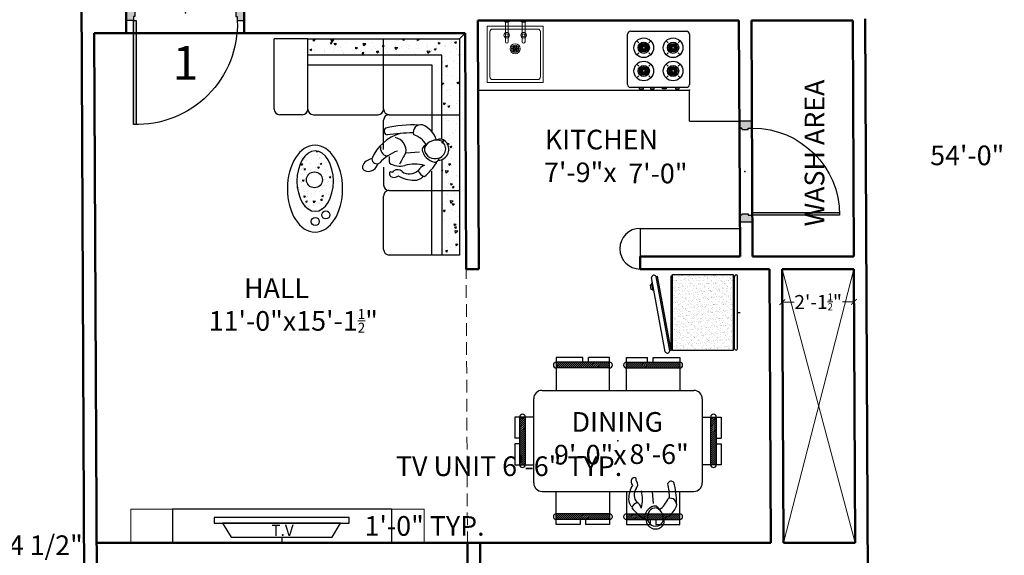
# Model space of a CAD drawing. Units: inches. Extents: x 4508 to 5907, y 877 to 1592.
# Tile 14 of 20: x 5553 to 5904, y 1107 to 1298. Entities that reach past the tile are written whole.
import ezdxf

# ---------------------------------------------------------------- set-up
doc = ezdxf.new("R2010")
doc.units = ezdxf.units.IN
doc.linetypes.add('DASHED', pattern=[0.75, 0.5, -0.25])
doc.layers.get('DEFPOINTS').update_dxf_attribs({"color": 8})
for name, color, linetype, lineweight in [('A-ANNO-DIMS', 2, 'Continuous', 18), ('A-ANNO-TEXT', 7, 'Continuous', 25), ('A-DOOR', 4, 'Continuous', 25), ('A-FLOR-CASE', 30, 'Continuous', 25), ('A-FLOR-FIXT', 8, 'Continuous', 18), ('A-FLOR-OVHD', 5, 'DASHED', 18), ('A-FLOR-SHFT', 8, 'Continuous', 18), ('A-FURN', 24, 'Continuous', 18), ('A-WALL', 7, 'Continuous', 50)]:
    doc.layers.add(name, color=color, linetype=linetype, lineweight=lineweight)
doc.layers.add('doors & windows', color=30, linetype='Continuous')
doc.layers.add('furniture', color=24, linetype='Continuous')
doc.styles.get("Standard").update_dxf_attribs({"font": 'arial.ttf'})
doc.dimstyles.new('details', dxfattribs={"dimtxt": 5, "dimasz": 2, "dimexe": 2, "dimexo": 3, "dimgap": 1, "dimtad": 0, "dimdec": 1, "dimzin": 0, "dimdsep": 46, "dimlunit": 4, "dimtxsty": 'Standard', "dimblk": 'ARCHTICK', "dimcen": 3, "dimclrd": 256, "dimclre": 256, "dimclrt": 256, "dimadec": 0, "dimazin": 0, "dimtfac": 0.5, "dimtdec": 1, "dimtofl": 0, "dimtmove": 0, "dimatfit": 3, "dimldrblk": 'CLOSEDBLANK', "dimfxl": 2, "dimtolj": 1, "dimtzin": 0, "dimlwd": -1, "dimlwe": -1, "dimarcsym": 0})
doc.dimstyles.new('text', dxfattribs={"dimtxt": 7, "dimasz": 0, "dimexe": 3, "dimexo": 3, "dimgap": 0, "dimtad": 1, "dimtih": 1, "dimtoh": 1, "dimzin": 3, "dimdsep": 46, "dimlunit": 4, "dimtxsty": 'Standard', "dimblk": 'CLOSEDBLANK', "dimcen": 3, "dimse1": 1, "dimse2": 1, "dimsd1": 1, "dimsd2": 1, "dimclrd": 256, "dimclre": 256, "dimclrt": 256, "dimadec": 0, "dimazin": 0, "dimtfac": 0.5, "dimtofl": 0, "dimtmove": 0, "dimatfit": 3, "dimfxl": 3, "dimtolj": 1, "dimtzin": 0, "dimlwd": -1, "dimlwe": -1, "dimarcsym": 0})
pattern_1 = [(45, (0, 0), (-0.3535534, 0.3535534), [])]

# ---------------------------------------------------------------- blocks, each defined once
blk = doc.blocks.new('MAN')
at = {"layer": 'doors & windows'}
blk.add_line((1.3, -9.85), (0.89, -5.45), dxfattribs=at)
for centre, radius, start, end in [((0.1, 0.48), 3.6, 2.8928, 134.5528), ((-0.36, -7.56), 8.07, 108.0153, 157.5724), ((-0.81, 1.3), 2.37, 132.7993, 210.1219), ((1.3, 0.05), 4.16, 155.2349, 248.5051), ((0, 0), 3.06, 359.7942, 144.0351), ((-0.98, 0.55), 5.34, 289.2819, 356.6237), ((2.86, -0.44), 1.38, 352.7443, 87.7525), ((-8.99, -19.77), 24.04, 41.647, 56.3067), ((4.14, -10.82), 9.46, 125.6851, 158.6987), ((0.38, -2.75), 1.79, 192.3382, 283.0231), ((-0.1, -0.61), 3.22, 267.7788, 10.6507), ((-5.32, -4.92), 2.54, 170.002, 284.7527), ((34.75, -7.19), 42.53, 177.9613, 192.4551), ((15.87, -7.04), 10.97, 162.7002, 196.7262), ((8.59, -3.01), 3.29, 193.5598, 239.9446), ((5.83, -2.73), 3.32, 289.6374, 341.2911), ((3.84, -8.67), 4.24, 325.4363, 41.8446), ((6.12, -7.03), 4.01, 358.2671, 46.939), ((54.76, -7.35), 59.95, 180.1044, 188.2297), ((-0.78, -6.94), 10.91, 330.7562, 358.8997), ((9.03, -7.36), 14.72, 197.1765, 246.7641), ((0.5, -14.05), 4.27, 79.2575, 168.509), ((12.84, -8.62), 12.77, 197.9012, 229.3504), ((16.49, 13.41), 27.78, 236.8487, 245.427), ((-0.19, -11.81), 5.78, 325.2412, 16.1794), ((8.85, -12.54), 2.12, 136.0875, 215.1077), ((7.06, -13.61), 2.15, 328.4119, 38.6474), ((3.21, -8.72), 6.53, 262.8142, 281.931), ((6.8, -14.37), 0.689, 315.9836, 61.7947), ((8.05, -14.12), 1.05, 224.0636, 323.687), ((-5.78, -15.61), 1.25, 217.214, 345.0614), ((-0.4, -15.27), 2.81, 261.6005, 345.5998), ((3.09, -19.2), 1.68, 274.444, 31.8659), ((4.09, -22.01), 3.16, 349.15, 77.9716), ((6.99, -20.36), 3.8, 187.9766, 248.0432), ((5.75, -22.44), 1.45, 262.6631, 353.5986)]:
    blk.add_arc(centre, radius, start, end, dxfattribs=at)
blk = doc.blocks.new('sofa 3')
at = {"layer": 'furniture', "ltscale": 0.5}
h = blk.add_hatch(dxfattribs=at)
h.set_pattern_fill('AR-CONC', color=256, angle=90, style=0)
h.set_pattern_definition([(220, (1099.1507, -871.655), (0.627521, -7.172602), [0.75, -8.25]), (275, (1099.151, -871.655), (-7.52192, 1.387513), [0.6, -6.6]), (169.5486, (1099.203, -872.253), (-6.894395, -5.785094), [0.637402, -7.01142]), (223.8158, (1097.151, -871.655), (1.65519, -10.67241), [1.125, -12.375]), (173.3644, (1097.289, -872.544), (-9.74118, -9.34663), [0.9561, -10.51713]), (278.8158, (1097.151, -871.655), (-9.74119, -9.34662), [0.9, -9.9]), (249, (1097.6507, -872.655), (4.02619, -5.96907), [0.75, -8.25]), (304, (1097.651, -872.655), (-7.2515, -2.433153), [0.6, -6.6]), (198.5486, (1097.986, -873.1524), (-3.225305, -8.402226), [0.637402, -7.01142]), (232.5, (1099.1507, -871.655), (-3.3289385, -0.1215986), [0, -6.52, 0, -6.7, 0, -6.625]), (262.5, (1099.1507, -871.655), (-3.944117, -2.630695), [0, -3.82, 0, -6.37, 0, -2.525]), (302.5, (1099.1507, -869.425), (0.2255487, -5.3382244), [0, -2.5, 0, -7.8, 0, -10.35]), (312.5, (1099.1507, -868.425), (-1.00105, -5.831862), [0, -3.25, 0, -5.18, 0, -7.35])])
h.paths.add_polyline_path([(2, 56), (2, 79), (8.27, 79), (8.27, 56)])
edge = h.paths.add_edge_path()
edge.add_arc((9.44, 36.7), 1.54, 139.4115, 177.7525)
edge.add_arc((8.94, 33.52), 3.4, 107.8673, 234.0351)
edge.add_arc((8.88, 34.97), 4.62, 245.2349, 262.3616)
edge.add_line((8.27, 30.38), (8.27, 29))
edge.add_line((8.27, 29), (2, 29))
edge.add_line((2, 29), (2, 56))
edge.add_line((2, 56), (8.27, 56))
edge.add_line((8.27, 56), (8.27, 37.7))
h.paths.add_polyline_path([(8.27, 7.77), (29, 7.77), (29, 2), (2, 2), (2, 29), (8.27, 29)])
h.paths.add_polyline_path([(29, 2), (29, 7.77), (56, 7.77), (56, 2)])
at = {"layer": 'furniture'}
h = blk.add_hatch(dxfattribs=at)
h.set_pattern_fill('AR-CONC', color=256, scale=0.8, angle=90, style=0)
h.set_pattern_definition([(220, (892.888, -686.9864), (0.502017, -5.738081), [0.6, -6.6]), (275, (892.888, -686.9864), (-6.017537, 1.11001), [0.48, -5.28]), (169.5486, (892.93, -687.4646), (-5.515516, -4.628075), [0.509922, -5.609137]), (223.8158, (891.288, -686.9864), (1.32415, -8.53793), [0.9, -9.9]), (173.3644, (891.3985, -687.698), (-7.79294, -7.4773), [0.76488, -8.413704]), (278.8158, (891.288, -686.986), (-7.79295, -7.477296), [0.72, -7.92]), (249, (891.688, -687.7864), (3.220951, -4.775256), [0.6, -6.6]), (304, (891.688, -687.7864), (-5.8012, -1.946523), [0.48, -5.28]), (198.5486, (891.9566, -688.1844), (-2.580244, -6.72178), [0.509922, -5.609137]), (232.5, (892.8881, -686.9864), (-2.663151, -0.097279), [0, -5.216, 0, -5.36, 0, -5.3]), (262.5, (892.8881, -686.9864), (-3.155294, -2.104556), [0, -3.056, 0, -5.096, 0, -2.02]), (302.5, (892.8881, -685.2024), (0.180439, -4.2705795), [0, -2, 0, -6.24, 0, -8.28]), (312.5, (892.888, -684.4024), (-0.80084, -4.665489), [0, -2.6, 0, -4.144, 0, -5.88])])
edge = h.paths.add_edge_path()
edge.add_ellipse((53.37, 52.67), major_axis=(0, 10.76), ratio=0.60396, start_angle=0, end_angle=360, ccw=False)
h.paths.add_polyline_path([(56.46, 52.22, -1), (50.81, 52.22, -1)], flags=16)
for p, q in [((2, 2), (2, 79)), ((2, 79), (27, 79)), ((8.27, 44.99), (8.27, 79)), ((11.8, 79), (11.8, 49.12)), ((29, 77), (29, 58)), ((27, 56), (2, 56)), ((29, 47.65), (29, 54)), ((29, 41.41), (29, 31)), ((8.27, 37.77), (8.27, 7.77)), ((11.8, 11.29), (11.8, 35.08)), ((8.27, 29), (2, 29)), ((27, 29), (8.27, 29)), ((54, 29), (31, 29)), ((58, 29), (66, 29)), ((29, 27), (29, 2)), ((56, 27), (56, 2)), ((68, 27), (68, 2)), ((56, 11.29), (11.8, 11.29)), ((8.27, 7.77), (56, 7.77)), ((2, 2), (0, 0)), ((56, 2), (2, 2)), ((56, 2), (68, 2))]:
    blk.add_line(p, q, dxfattribs=at)
for centre, radius in [((53.36, 67.05), 1.44), ((49.58, 64.71), 1.44), ((53.63, 52.22), 2.83)]:
    blk.add_circle(centre, radius, dxfattribs=at)
for centre, start, end in [((27, 77), 0, 90), ((27, 58), 270, 0), ((27, 54), 0, 90), ((27, 31), 270, 0), ((27, 27), 0, 90), ((31, 27), 90, 180), ((54, 27), 0, 90), ((58, 27), 90, 180), ((66, 27), 0, 90)]:
    blk.add_arc(centre, 2, start, end, dxfattribs=at)
at = {"layer": 'furniture', "extrusion": (0, 0, -1)}
for centre, major_axis, ratio in [((53.43, 55.37), (0, 15.49), 0.635514), ((53.37, 52.67), (0, 10.76), 0.60396)]:
    blk.add_ellipse(centre, major_axis=major_axis, ratio=ratio, dxfattribs=at)
at = {"xscale": 1.1, "yscale": 1.1, "zscale": 1.1, "rotation": 90}
blk.add_blockref('MAN', (10.27, 41.21), dxfattribs=at)
blk = doc.blocks.new('MD')
at = {"layer": 'doors & windows'}
h = blk.add_hatch(dxfattribs=at)
h.set_pattern_fill('DOTS', color=256, scale=2, style=0)
h.set_pattern_definition([(180, (0, -4), (-0.0625, 0.125), [0, -0.125])])
h.paths.add_polyline_path([(2.5, 37), (3.5, 37), (3.5, 0), (2.5, 0)])
h = blk.add_hatch(dxfattribs=at)
h.set_pattern_fill('DOTS', color=256, scale=2, style=0)
h.set_pattern_definition([(0, (0, -0.5), (0.0625, 0.125), [0, -0.125])])
h.paths.add_polyline_path([(42, -4.5), (42, 0), (39.5, 0), (39.5, -1.5), (39, -1.5), (39, -3.75), (39.25, -3.75, 0.403966), (39.75, -4.25), (39.75, -4.5)])
h.paths.add_polyline_path([(0, -4.5), (2.25, -4.5), (2.25, -4.25, 0.403966), (2.75, -3.75), (3, -3.75), (3, -1.5), (2.5, -1.5), (2.5, 0), (0, 0)])
for p, q in [((0, 0), (0, -4.5)), ((42, 0), (42, -4.5))]:
    blk.add_line(p, q)
blk.add_line((0, -4.5), (2.25, -4.5), dxfattribs=at)
blk.add_lwpolyline([(3.5, 0), (3.5, 37), (2.5, 37), (2.5, 0)], close=True, dxfattribs=at)
for points in [[(3, -3.75), (3, -1.5), (2.5, -1.5), (2.5, 0), (0, 0)], [(39, -3.75), (39, -1.5), (39.5, -1.5), (39.5, 0), (42, 0)], [(42, -4.5), (39.75, -4.5)]]:
    blk.add_lwpolyline(points, dxfattribs=at)
for points in [[(2.25, -4.5), (2.25, -4.25, 0.403966), (2.75, -3.75), (3, -3.75)], [(39.75, -4.5), (39.75, -4.25, -0.403966), (39.25, -3.75), (39, -3.75)]]:
    blk.add_lwpolyline(points, format="xyb", dxfattribs=at)
at = {"layer": 'doors & windows', "ltscale": 6}
blk.add_arc((3.73, 1.23), 35.79, 358.0281, 91.9719, dxfattribs=at)
at = {"layer": 'doors & windows'}
blk.add_point((21, -2.75), dxfattribs=at)
blk = doc.blocks.new('*D127')
at = {"layer": 'DEFPOINTS', "color": 0, "transparency": 16777216}
for p in [(5656.84, 1293.42), (5666.22, 1293.42), (5644.05, 1111.92)]:
    blk.add_point(p, dxfattribs=at)
at = {"layer": 'A-ANNO-DIMS', "color": 0, "transparency": 16777216, "insert": (5666.22, 1190.97), "char_height": 7, "attachment_point": 5}
blk.add_mtext('\\A1;15\'-1{\\H0.5x;\\S1/2;}"', dxfattribs=at)
blk = doc.blocks.new('_ClosedBlank')
at = {"color": 0, "lineweight": -2}
for p, q in [((-1, 0.17), (0, 0)), ((-1, 0.17), (-1, -0.17)), ((0, 0), (-1, -0.17))]:
    blk.add_line(p, q, dxfattribs=at)
blk = doc.blocks.new('*D128')
at = {"layer": 'DEFPOINTS', "color": 0, "transparency": 16777216}
for p in [(5712.25, 1194.15), (5580.27, 1189.78), (5712.25, 1187.38)]:
    blk.add_point(p, dxfattribs=at)
at = {"layer": 'A-ANNO-DIMS', "color": 0, "transparency": 16777216, "insert": (5636.1, 1196.78), "char_height": 7, "attachment_point": 5}
blk.add_mtext('\\A1;        HALL\\P11\'-0"x', dxfattribs=at)
blk = doc.blocks.new('tv')
at = {"layer": 'furniture'}
blk.add_line((0, 0), (2, 0), dxfattribs=at)
for points in [[(0, -39), (12, -39), (12, 39), (0, 39)], [(7, 24.19), (7, -23.81), (9, -23.81), (9, 24.19), (7, 24.19)]]:
    blk.add_lwpolyline(points, dxfattribs=at)
blk.add_lwpolyline([(7, -20.81), (7, 21.19), (2, 18.19), (2, -17.81)], close=True, dxfattribs=at)
blk.add_text('T.V', height=4, rotation=270, dxfattribs=at).set_placement((2.46, 3.81))
blk = doc.blocks.new('D1')
at = {"layer": 'doors & windows'}
h = blk.add_hatch(dxfattribs=at)
h.set_pattern_fill('DOTS', color=256, scale=2, angle=180, style=0)
h.set_pattern_definition([(180, (-2e-12, -4), (-0.0625, -0.125), [0, -0.125])])
h.paths.add_polyline_path([(2.5, 0), (3.5, 0), (3.5, 30.98, 0.008066), (2.5, 31)])
h = blk.add_hatch(dxfattribs=at)
h.set_pattern_fill('DOTS', color=256, scale=2, angle=180, style=0)
h.set_pattern_definition([(180, (0, -0.5), (-0.0625, -0.125), [0, -0.125])])
h.paths.add_polyline_path([(0, -4.5), (2.25, -4.5), (2.25, -4.25, 0.403966), (2.75, -3.75), (3, -3.75), (3, -1.5), (2.5, -1.5), (2.5, 0), (0, 0)])
h.paths.add_polyline_path([(36, -4.5), (36, 0), (33.5, 0), (33.5, -1.5), (33, -1.5), (33, -3.75), (33.25, -3.75, 0.403966), (33.75, -4.25), (33.75, -4.5)])
for p, q in [((0, 0), (0, -4.5)), ((36, 0), (36, -4.5))]:
    blk.add_line(p, q)
blk.add_lwpolyline([(3.5, 0), (3.5, 31), (2.5, 31), (2.5, 0)], close=True, dxfattribs=at)
for points in [[(3, -3.75), (3, -1.5), (2.5, -1.5), (2.5, 0), (0, 0)], [(33, -3.75), (33, -1.5), (33.5, -1.5), (33.5, 0), (36, 0)], [(0, -4.5), (2.25, -4.5)], [(36, -4.5), (33.75, -4.5)]]:
    blk.add_lwpolyline(points, dxfattribs=at)
for points in [[(2.25, -4.5), (2.25, -4.25, 0.403966), (2.75, -3.75), (3, -3.75)], [(33.75, -4.5), (33.75, -4.25, -0.403966), (33.25, -3.75), (33, -3.75)]]:
    blk.add_lwpolyline(points, format="xyb", dxfattribs=at)
at = {"layer": 'doors & windows', "ltscale": 6}
blk.add_arc((2.5, 0), 31, 0, 90, dxfattribs=at)
at = {"layer": 'doors & windows'}
blk.add_point((18, -2.75), dxfattribs=at)
blk = doc.blocks.new('*D129')
at = {"layer": 'DEFPOINTS', "color": 0, "transparency": 16777216}
for p in [(5716.62, 1265.12), (5809.62, 1261.37), (5809.62, 1240.24)]:
    blk.add_point(p, dxfattribs=at)
at = {"layer": 'A-ANNO-DIMS', "color": 0, "transparency": 16777216, "insert": (5752.82, 1249.71), "char_height": 7, "attachment_point": 5}
blk.add_mtext('\\A1;       KITCHEN\\P7\'-9"x', dxfattribs=at)
blk = doc.blocks.new('*D130')
at = {"layer": 'DEFPOINTS', "color": 0, "transparency": 16777216}
for p in [(5755.88, 1295.12), (5780.42, 1295.12), (5782.03, 1211.12)]:
    blk.add_point(p, dxfattribs=at)
at = {"layer": 'A-ANNO-DIMS', "color": 0, "transparency": 16777216, "insert": (5780.42, 1243.47), "char_height": 7, "attachment_point": 5}
blk.add_mtext('\\A1;7\'-0"', dxfattribs=at)
blk = doc.blocks.new('stove')
at = {"layer": 'furniture'}
h = blk.add_hatch(dxfattribs=at)
h.set_pattern_fill('HEX', color=256, angle=180, style=0)
h.set_pattern_definition([(360, (22, 21.5), (1e-16, 0.2165064), [0.125, -0.25]), (120, (22, 21.5), (-0.1875, -0.1082532), [0.125, -0.25]), (60, (22.125, 21.5), (-0.1875, 0.1082532), [0.125, -0.25])])
h.paths.add_polyline_path([(5.36, 16.21, 1), (8.36, 16.21, 1)])
h.paths.add_polyline_path([(7.36, 16.21, -1), (6.36, 16.21, -1)], flags=16)
h = blk.add_hatch(dxfattribs=at)
h.set_pattern_fill('HEX', color=256, angle=180, style=0)
h.set_pattern_definition([(180, (2e-13, 21.5), (-1e-16, 0.2165064), [0.125, -0.25]), (60, (2e-13, 21.5), (0.1875, -0.1082532), [0.125, -0.25]), (120, (-0.125, 21.5), (0.1875, 0.1082532), [0.125, -0.25])])
h.paths.add_polyline_path([(13.64, 16.21, 1), (16.64, 16.21, 1)])
h.paths.add_polyline_path([(15.64, 16.21, -1), (14.64, 16.21, -1)], flags=16)
h = blk.add_hatch(dxfattribs=at)
h.set_pattern_fill('HEX', color=256, angle=180, style=0)
h.set_pattern_definition([(360, (22, 0.5), (-1e-16, -0.2165064), [0.125, -0.25]), (240, (22, 0.5), (-0.1875, 0.1082532), [0.125, -0.25]), (300, (22.125, 0.5), (-0.1875, -0.1082532), [0.125, -0.25])])
h.paths.add_polyline_path([(8.36, 5.79, 1), (5.36, 5.79, 1)])
h.paths.add_polyline_path([(6.36, 5.79, -1), (7.36, 5.79, -1)], flags=16)
h = blk.add_hatch(dxfattribs=at)
h.set_pattern_fill('HEX', color=256, angle=180, style=0)
h.set_pattern_definition([(180, (2e-13, 0.5), (1e-16, -0.2165064), [0.125, -0.25]), (300, (2e-13, 0.5), (0.1875, 0.1082532), [0.125, -0.25]), (240, (-0.125, 0.5), (0.1875, -0.1082532), [0.125, -0.25])])
h.paths.add_polyline_path([(16.64, 5.79, 1), (13.64, 5.79, 1)])
h.paths.add_polyline_path([(14.64, 5.79, -1), (15.64, 5.79, -1)], flags=16)
for p, q in [((2, 22), (20, 22)), ((1, 17.86), (0.5, 17.86)), ((0.5, 17.86), (0.5, 16.36)), ((1, 1), (1, 21)), ((4.39, 18.69), (5.1, 17.98)), ((8.63, 17.98), (9.34, 18.69)), ((13.37, 17.98), (12.66, 18.69)), ((17.61, 18.69), (16.9, 17.98)), ((21, 21), (21, 1)), ((0.5, 16.36), (1, 16.36)), ((4.39, 13.74), (5.1, 14.45)), ((8.63, 14.45), (9.34, 13.74)), ((13.37, 14.45), (12.66, 13.74)), ((17.61, 13.74), (16.9, 14.45)), ((0.5, 13.8), (0.5, 12.5)), ((1, 13.8), (0.5, 13.8)), ((0.5, 12.5), (1, 12.5)), ((0.5, 9.5), (1, 9.5)), ((0.5, 8.2), (0.5, 9.5)), ((1, 8.2), (0.5, 8.2)), ((4.39, 8.26), (5.1, 7.55)), ((8.63, 7.55), (9.34, 8.26)), ((13.37, 7.55), (12.66, 8.26)), ((17.61, 8.26), (16.9, 7.55)), ((0.5, 4.94), (0.5, 3.64)), ((1, 4.94), (0.5, 4.94)), ((0.5, 3.64), (1, 3.64)), ((4.39, 3.31), (5.1, 4.02)), ((8.63, 4.02), (9.34, 3.31)), ((13.37, 4.02), (12.66, 3.31)), ((17.61, 3.31), (16.9, 4.02)), ((20, 0), (2, 0))]:
    blk.add_line(p, q, dxfattribs=at)
for centre, radius in [((6.86, 16.21), 3.5), ((6.86, 16.21), 2), ((6.86, 16.21), 1.5), ((15.14, 16.21), 3.5), ((15.14, 16.21), 2), ((15.14, 16.21), 1.5), ((6.86, 16.21), 0.5), ((15.14, 16.21), 0.5), ((6.86, 5.79), 3.5), ((6.86, 5.79), 2), ((6.86, 5.79), 1.5), ((15.14, 5.79), 3.5), ((15.14, 5.79), 2), ((15.14, 5.79), 1.5), ((6.86, 5.79), 0.5), ((15.14, 5.79), 0.5)]:
    blk.add_circle(centre, radius, dxfattribs=at)
for centre, start, end in [((2, 21), 90, 180), ((20, 21), 0, 90), ((2, 1), 180, 270), ((20, 1), 270, 0)]:
    blk.add_arc(centre, 1, start, end, dxfattribs=at)
at = {"layer": 'furniture', "ltscale": 9}
blk.add_point((0, 0), dxfattribs=at)
blk = doc.blocks.new('sink')
for p, q in [((0, 0), (-24, 0)), ((0, 0), (0, 0)), ((-22, -3), (-2, -3)), ((-22, -23), (-22, -3)), ((-2, -3), (-2, -23)), ((-21, -21), (-21, -5)), ((-20, -4), (-4, -4)), ((-3, -5), (-3, -21)), ((-0.5, -9.5), (-7.5, -9.5)), ((-0.5, -10.5), (-7.5, -10.5)), ((-0.5, -9.5), (-0.5, -10.5)), ((0, -9), (0, -11)), ((-0.5, -15.5), (-7.5, -15.5)), ((-0.5, -16.5), (-7.5, -16.5)), ((-0.5, -15.5), (-0.5, -16.5)), ((0, -15), (0, -17)), ((-22, -23), (-2, -23)), ((-20, -22), (-4, -22))]:
    blk.add_line(p, q)
for centre, radius in [((-5.18, -10), 1), ((-5.18, -10), 0.5), ((-10, -13), 1.79), ((-10, -13), 1.29), ((-10.66, -12.62), 0.25), ((-10.66, -13.38), 0.25), ((-10, -12.24), 0.25), ((-10, -13), 0.25), ((-10, -13.76), 0.25), ((-9.34, -12.62), 0.25), ((-9.34, -13.38), 0.25), ((-5.18, -16), 1), ((-5.18, -16), 0.5)]:
    blk.add_circle(centre, radius)
for centre, radius, start, end in [((-20, -5), 1, 90, 180), ((-4, -5), 1, 0, 90), ((-7.5, -10), 0.5, 90, 270), ((0.01, -9.51), 0.511, 91.1728, 178.8272), ((0.01, -10.49), 0.511, 181.1728, 268.8272), ((-7.5, -16), 0.5, 90, 270), ((0.01, -15.51), 0.511, 91.1728, 178.8272), ((0.01, -16.49), 0.511, 181.1728, 268.8272), ((-20, -21), 1, 180, 270), ((-4, -21), 1, 270, 0)]:
    blk.add_arc(centre, radius, start, end)
blk = doc.blocks.new('*D131')
at = {"layer": 'DEFPOINTS', "color": 0, "transparency": 16777216}
for p in [(5712.47, 1147.27), (5820.46, 1147.91), (5712.47, 1139.67)]:
    blk.add_point(p, dxfattribs=at)
at = {"layer": 'A-ANNO-DIMS', "color": 0, "transparency": 16777216, "insert": (5756.37, 1149.13), "char_height": 7, "attachment_point": 5}
blk.add_mtext('\\A1;         DINING\\P9\'-0"x', dxfattribs=at)
blk = doc.blocks.new('*D132')
at = {"layer": 'DEFPOINTS', "color": 0, "transparency": 16777216}
for p in [(5771.01, 1205.73), (5780.86, 1205.73), (5764.79, 1103.73)]:
    blk.add_point(p, dxfattribs=at)
at = {"layer": 'A-ANNO-DIMS', "color": 0, "transparency": 16777216, "insert": (5780.86, 1143.5), "char_height": 7, "attachment_point": 5}
blk.add_mtext('\\A1;8\'-6"', dxfattribs=at)
blk = doc.blocks.new('DT')
at = {"layer": 'furniture'}
h = blk.add_hatch(dxfattribs=at)
h.set_pattern_fill('ANSI31', color=256, scale=4, style=0)
h.set_pattern_definition(pattern_1)
h.paths.add_polyline_path([(-34, -8.5), (-32, -8.5), (-32, 8.5), (-34, 8.5)])
h.paths.add_polyline_path([(-2, 26), (-2, 28), (-21, 28), (-21, 26)])
h.paths.add_polyline_path([(23, 26), (23, 28), (4, 28), (4, 26)])
h.paths.add_polyline_path([(23, -28), (23, -26), (4, -26), (4, -28)])
h.paths.add_polyline_path([(-2, -28), (-2, -26), (-21, -26), (-21, -28)])
h = blk.add_hatch(dxfattribs=at)
h.set_pattern_fill('ANSI31', color=256, scale=4, style=0)
h.set_pattern_definition(pattern_1)
h.paths.add_polyline_path([(34, -8.5), (36, -8.5), (36, 8.5), (34, 8.5)])
at = {"layer": 'doors & windows'}
blk.add_line((-11.2, 18.15), (-11.59, 22.33), dxfattribs=at)
for centre, radius, start, end in [((-13.21, 28.75), 2.25, 132.7993, 210.1219), ((-11.2, 27.56), 3.95, 155.2349, 248.5051), ((-12.43, 27.51), 2.91, 359.7942, 144.0351), ((-12.34, 27.96), 3.42, 2.8928, 134.5528), ((-9.72, 27.09), 1.31, 352.7443, 87.7525), ((-12.78, 20.33), 7.67, 108.0153, 157.5724), ((-12.53, 26.93), 3.05, 267.7788, 10.6507), ((-13.37, 28.03), 5.08, 289.2819, 356.6237), ((-20.97, 8.73), 22.84, 41.647, 56.3067), ((-17.49, 22.83), 2.42, 170.002, 284.7527), ((1.32, 21.08), 21.14, 177.1977, 197.248), ((-8.5, 17.23), 8.99, 125.6851, 158.6987), ((-12.08, 24.9), 1.7, 192.3382, 283.0231), ((2.64, 20.82), 10.42, 162.7002, 196.7262), ((-4.27, 24.65), 3.12, 193.5598, 239.9446), ((-6.9, 24.92), 3.16, 289.6374, 341.2911), ((-8.79, 19.27), 4.03, 325.4363, 41.8446), ((-6.62, 20.83), 3.81, 358.2671, 46.939), ((6.61, 20.49), 23.98, 180.1725, 192.6992), ((-13.17, 20.91), 10.36, 330.7562, 358.8997), ((-17.93, 15.53), 1.19, 217.214, 345.0614), ((-4.02, 15.59), 2.01, 136.0875, 215.1077), ((-5.98, 13.86), 0.655, 315.9836, 61.7947), ((-5.73, 14.57), 2.04, 328.4119, 38.6474), ((-4.79, 14.1), 0.998, 224.0636, 323.687)]:
    blk.add_arc(centre, radius, start, end, dxfattribs=at)
at = {"layer": 'furniture'}
for p, q in [((-21, 29.75), (-21, 18)), ((-12.5, 29.75), (-21, 29.75)), ((-12.5, 28), (-12.5, 29.75)), ((-10.5, 28), (-10.5, 29.75)), ((-2, 29.75), (-10.5, 29.75)), ((-2, 18), (-2, 29.75)), ((4, 18), (4, 29.75)), ((4, 29.75), (12.5, 29.75)), ((12.5, 28), (12.5, 29.75)), ((14.5, 28), (14.5, 29.75)), ((14.5, 29.75), (23, 29.75)), ((23, 29.75), (23, 18)), ((-2, 28), (-21, 28)), ((-2, 26), (-21, 26)), ((4, 28), (23, 28)), ((4, 26), (23, 26)), ((28, 18), (-26, 18)), ((-29, -15), (-29, 15)), ((31, 15), (31, -15)), ((-35.75, 1), (-35.75, 8.5)), ((-35.75, 8.5), (-29, 8.5)), ((-34, -8.5), (-34, 8.5)), ((-32, -8.5), (-32, 8.5)), ((37.75, 8.5), (31, 8.5)), ((34, -8.5), (34, 8.5)), ((36, -8.5), (36, 8.5)), ((37.75, 1), (37.75, 8.5)), ((-34, 1), (-35.75, 1)), ((36, 1), (37.75, 1)), ((-34, -1), (-35.75, -1)), ((-35.75, -8.5), (-35.75, -1)), ((36, -1), (37.75, -1)), ((37.75, -8.5), (37.75, -1)), ((-29, -8.5), (-35.75, -8.5)), ((31, -8.5), (37.75, -8.5)), ((28, -18), (-26, -18)), ((-21, -29.75), (-21, -18)), ((-2, -18), (-2, -29.75)), ((4, -18), (4, -29.75)), ((23, -29.75), (23, -18)), ((-2, -26), (-21, -26)), ((-2, -28), (-21, -28)), ((-11.5, -28), (-11.5, -29.75)), ((-9.5, -28), (-9.5, -29.75)), ((4, -26), (23, -26)), ((4, -28), (23, -28)), ((11.5, -28), (11.5, -29.75)), ((13.5, -28), (13.5, -29.75)), ((-11.5, -29.75), (-21, -29.75)), ((-2, -29.75), (-9.5, -29.75)), ((4, -29.75), (11.5, -29.75)), ((13.5, -29.75), (23, -29.75))]:
    blk.add_line(p, q, dxfattribs=at)
for centre, radius, start, end in [((-21, 27), 1, 90, 270), ((-2, 27), 1, 270, 90), ((4, 27), 1, 90, 270), ((23, 27), 1, 270, 90), ((-26, 15), 3, 90, 180), ((28, 15), 3, 0, 90), ((-33, 8.5), 1, 0, 180), ((35, 8.5), 1, 0, 180), ((-33, -8.5), 1, 180, 0), ((35, -8.5), 1, 180, 0), ((-26, -15), 3, 180, 270), ((28, -15), 3, 270, 0), ((-21, -27), 1, 90, 270), ((-2, -27), 1, 270, 90), ((4, -27), 1, 90, 270), ((23, -27), 1, 270, 90)]:
    blk.add_arc(centre, radius, start, end, dxfattribs=at)
blk.add_point((1, 0), dxfattribs=at)
blk = doc.blocks.new('refrigerator')
at = {"layer": 'furniture'}
h = blk.add_hatch(dxfattribs=at)
h.set_pattern_fill('AR-SAND', color=256, angle=-90, style=0)
h.set_pattern_definition([(307.5, (-13.5104, -1), (1.926824, 0.06299), [0, -1.52, 0, -1.7, 0, -1.625]), (277.5, (-13.5104, -1), (2.82215, -1.76978), [0, -0.82, 0, -1.37, 0, -0.525]), (237.5, (-13.5104, 0.23), (0.00566, -3.11414), [0, -0.5, 0, -1.8, 0, -2.35]), (227.5, (-13.5104, 0.23), (0.87768, -3.00613), [0, -0.25, 0, -1.18, 0, -1.35])])
h.paths.add_polyline_path([(13.6, -24.16), (13.6, -2.56), (-13.51, -2.56), (-13.51, -24.16)])
for p, q in [((0, -1), (0, 0)), ((-13.51, -2.56), (13.6, -2.56)), ((-13.51, -24.16), (-13.51, -2.56)), ((12.94, -1), (-12.94, -1)), ((12.94, -2), (-12.94, -2)), ((-12.41, -2), (-12.41, -2.56)), ((12.29, -2), (12.29, -2.56)), ((13.6, -2.56), (13.6, -24.16)), ((13.6, -24.16), (-13.51, -24.16)), ((-13.07, -24.59), (-13.07, -24.16)), ((13.26, -24.59), (13.26, -24.16)), ((13.26, -24.59), (-13.07, -24.59)), ((13.6, -24.61), (-12.95, -29.5)), ((13.7, -25.1), (-12.85, -29.99)), ((14.06, -26.73), (-12.49, -31.62)), ((13.07, -24.59), (13.26, -24.62)), ((13.26, -24.62), (13.07, -24.71)), ((13.6, -24.61), (13.7, -25.1)), ((-12.85, -29.99), (-12.95, -29.5)), ((-10.58, -31.27), (-10.49, -31.65)), ((-10.49, -31.65), (-7.79, -31.16)), ((-8.23, -31.24), (-8.13, -31.69)), ((-7.79, -31.16), (-7.88, -30.77)), ((-9.87, -32.01), (-9.97, -31.56)), ((-8.13, -31.69), (-9.87, -32.01))]:
    blk.add_line(p, q, dxfattribs=at)
for centre, radius, start, end in [((-12.94, -1.5), 0.5, 90, 270), ((12.94, -1.5), 0.5, 270, 90), ((13.58, -25.98), 0.888, 302.2332, 82.2568), ((-12.38, -30.74), 0.888, 122.2332, 262.2568)]:
    blk.add_arc(centre, radius, start, end, dxfattribs=at)
blk = doc.blocks.new('_ArchTick')
at = {"color": 0, "linetype": 'ByBlock', "const_width": 0.15}
blk.add_lwpolyline([(-0.5, -0.5), (0.5, 0.5)], dxfattribs=at)
blk = doc.blocks.new('*D133')
at = {"layer": 'A-ANNO-DIMS', "color": 0, "transparency": 16777216}
for p, q in [((5824.69, 1206.3), (5824.74, 1195.64)), ((5850.19, 1206.42), (5850.24, 1195.76)), ((5824.73, 1197.64), (5828.88, 1197.66)), ((5850.23, 1197.76), (5846.08, 1197.74))]:
    blk.add_line(p, q, dxfattribs=at)
at = {"layer": 'DEFPOINTS', "color": 0, "transparency": 16777216}
for p in [(5824.68, 1209.3), (5850.18, 1209.42), (5850.23, 1197.76)]:
    blk.add_point(p, dxfattribs=at)
at = {"layer": 'A-ANNO-DIMS', "color": 0, "transparency": 16777216, "xscale": 2, "yscale": 2, "zscale": 2}
for p, rotation in [((5824.73, 1197.64), 180.2652563433842), ((5850.23, 1197.76), 0.2652563433842005)]:
    blk.add_blockref('_ArchTick', p, dxfattribs=dict(at, rotation=rotation))
at = {"layer": 'A-ANNO-DIMS', "color": 0, "transparency": 16777216, "insert": (5837.48, 1197.7), "char_height": 5, "attachment_point": 5, "rotation": 0.2653}
blk.add_mtext('\\A1;2\'-1{\\H0.5x;\\S1/2;}"', dxfattribs=at)
blk = doc.blocks.new('*D166')
at = {"layer": 'DEFPOINTS', "color": 0, "transparency": 16777216}
for p in [(5607.66, 1135.62), (5607.66, 1123.92), (5685.66, 1123.92)]:
    blk.add_point(p, dxfattribs=at)
at = {"layer": 'A-ANNO-DIMS', "transparency": 16777216, "insert": (5727.45, 1139.19), "char_height": 7, "attachment_point": 5}
blk.add_mtext('\\A1;TV UNIT 6\'-6" TYP.', dxfattribs=at)
blk = doc.blocks.new('*D167')
at = {"layer": 'DEFPOINTS', "color": 0, "transparency": 16777216}
for p in [(5685.66, 1123.92), (5697.36, 1123.92), (5685.66, 1111.92)]:
    blk.add_point(p, dxfattribs=at)
at = {"layer": 'A-ANNO-DIMS', "transparency": 16777216, "insert": (5697.36, 1117.92), "char_height": 7, "attachment_point": 5}
blk.add_mtext('\\A1;1\'-0" TYP.', dxfattribs=at)
blk = doc.blocks.new('*D191')
at = {"layer": 'DEFPOINTS', "color": 0, "transparency": 16777216}
for p in [(5539.438529, 1302.416611), (5579.745522, 1302.416611), (5579.787188, 1293.416611)]:
    blk.add_point(p, dxfattribs=at)
at = {"layer": 'A-ANNO-DIMS', "transparency": 16777216, "insert": (5539.438529, 1297.916611), "char_height": 7, "attachment_point": 5}
blk.add_mtext('\\A1;0\'-9"', dxfattribs=at)
blk = doc.blocks.new('*D193')
at = {"layer": 'DEFPOINTS', "color": 0, "transparency": 16777216}
for p in [(5539.44, 1111.92), (5580.63, 1111.92), (5580.65, 1107.42)]:
    blk.add_point(p, dxfattribs=at)
at = {"layer": 'A-ANNO-DIMS', "transparency": 16777216, "insert": (5556.9, 1111.04), "char_height": 7, "attachment_point": 5}
blk.add_mtext('\\A1;0\'-4 1/2"', dxfattribs=at)
blk = doc.blocks.new('*D194')
at = {"layer": 'DEFPOINTS', "color": 0, "transparency": 16777216}
for p in [(5854.266243, 1573.916611), (5890.541519, 1573.916611), (5855.991519, 925.916611)]:
    blk.add_point(p, dxfattribs=at)
at = {"layer": 'A-ANNO-DIMS', "transparency": 16777216, "insert": (5890.541519, 1249.916611), "char_height": 7, "attachment_point": 5}
blk.add_mtext('\\A1;54\'-0"', dxfattribs=at)

msp = doc.modelspace()

# ---------------------------------------------------------------- linework, layer by layer
at = {"layer": 'A-FLOR-CASE'}
for p, q in [((5716.383, 1273.119), (5791.615, 1273.119)), ((5791.615, 1262.119), (5791.615, 1273.119)), ((5791.615, 1262.119), (5809.435, 1262.119)), ((5774.101, 1223.917), (5809.658, 1223.917)), ((5774.101, 1223.917), (5774.101, 1213.917))]:
    msp.add_line(p, q, dxfattribs=at)
msp.add_arc((5774.101, 1216.667), 7.25, 90, 270, dxfattribs=at)
at = {"layer": 'A-FLOR-OVHD', "ltscale": 9}
msp.add_line((5712.631, 1111.417), (5712.178, 1209.396), dxfattribs=at)
at = {"layer": 'A-FLOR-SHFT', "ltscale": 9}
for p, q in [((5850.63, 1111.917), (5824.679, 1209.417)), ((5825.13, 1111.917), (5850.179, 1209.417))]:
    msp.add_line(p, q, dxfattribs=at)
at = {"layer": 'A-FURN'}
msp.add_lwpolyline([(5697.227, 1111.917), (5697.227, 1123.917), (5592.827, 1123.917), (5592.827, 1111.917)], dxfattribs=at)
at = {"layer": 'A-WALL'}
for p, q in [((5576.989, 925.917), (5573.989, 1573.917)), ((5591.171, 1293.417), (5591.171, 1302.417)), ((5633.198, 1302.417), (5633.198, 1293.417)), ((5716.678, 1209.417), (5716.268, 1297.937)), ((5716.268, 1297.917), (5809.269, 1297.917)), ((5809.658, 1213.917), (5809.269, 1297.917)), ((5813.769, 1297.917), (5849.769, 1297.917)), ((5814.158, 1213.917), (5813.769, 1297.917)), ((5850.158, 1213.917), (5849.769, 1297.917)), ((5855.992, 925.917), (5854.266, 1298.576)), ((5579.746, 1293.417), (5711.789, 1293.417)), ((5581.148, 999.417), (5579.787, 1293.417)), ((5712.178, 1209.396), (5711.789, 1293.417)), ((5774.101, 1213.917), (5809.658, 1213.917)), ((5774.101, 1213.917), (5774.101, 1209.417)), ((5814.158, 1213.917), (5850.158, 1213.917)), ((5716.678, 1209.417), (5712.178, 1209.396)), ((5774.101, 1209.417), (5820.179, 1209.417)), ((5820.63, 1111.917), (5820.179, 1209.417)), ((5825.13, 1111.917), (5824.679, 1209.417)), ((5824.679, 1209.417), (5850.179, 1209.417)), ((5850.63, 1111.917), (5850.179, 1209.417)), ((5580.627, 1111.917), (5820.63, 1111.917)), ((5713.15, 999.417), (5712.629, 1111.917)), ((5717.969, 930.417), (5717.129, 1111.917)), ((5825.13, 1111.917), (5850.63, 1111.917))]:
    msp.add_line(p, q, dxfattribs=at)

# ---------------------------------------------------------------- block references
at = {"layer": 'A-DOOR', "xscale": -1}
for name, p, rotation in [('MD', (5591.198, 1297.931), 180), ('D1', (5814.115, 1226.119), 270)]:
    msp.add_blockref(name, p, dxfattribs=dict(at, rotation=rotation))
at = {"layer": 'A-FLOR-FIXT'}
for name, p, rotation in [('sink', (5716.615, 1297.917), 90), ('stove', (5791.615, 1273.119), 90), ('refrigerator', (5809.75, 1193.965), 270)]:
    msp.add_blockref(name, p, dxfattribs=dict(at, rotation=rotation))
at = {"layer": 'A-FURN'}
for name, p, rotation in [('sofa 3', (5711.789, 1293.417), 180), ('DT', (5767.203, 1148.216), 180), ('tv', (5646.655, 1111.917), 90)]:
    msp.add_blockref(name, p, dxfattribs=dict(at, rotation=rotation))

# ---------------------------------------------------------------- texts
at = {"layer": 'A-ANNO-TEXT'}
msp.add_text('1', height=12, dxfattribs=at).set_placement((5607.729, 1276.89))
msp.add_text('WASH AREA', height=7, rotation=90, dxfattribs=at).set_placement((5839.678, 1224.619))

# ---------------------------------------------------------------- dimensions: what is measured, and where the dimension line sits
at = {"layer": 'A-ANNO-DIMS'}
for base, p1, p2, picture, middle in [((5890.542, 1573.917), (5855.992, 925.917), (5854.266, 1573.917), '*D194', (5890.542, 1249.917)), ((5539.439, 1302.417), (5579.787, 1293.417), (5579.746, 1302.417), '*D191', (5539.439, 1297.917)), ((5539.439, 1111.917), (5580.648, 1107.417), (5580.627, 1111.917), '*D193', (5556.898, 1111.036))]:
    dim = msp.add_linear_dim(base=base, p1=p1, p2=p2, angle=90, dimstyle='text', override={"dimdec": 1, "dimlfac": 1, "dimrnd": 0, "dimzin": 1, "dimdsep": 46, "dimlunit": 4, "dimfrac": 2}, dxfattribs=at)
    dim.commit()
    dim.dimension.update_dxf_attribs({"geometry": picture, "text_midpoint": middle})
for base, p1, p2, override, picture, middle in [((5666.22, 1293.417), (5644.053, 1111.917), (5656.843, 1293.417), {"dimtad": 0, "dimclrd": 0, "dimclre": 0, "dimclrt": 0}, '*D127', (5666.22, 1190.973)), ((5780.422, 1295.119), (5782.034, 1211.119), (5755.879, 1295.119), {"dimclrd": 0, "dimclre": 0, "dimclrt": 0}, '*D130', (5780.422, 1243.473)), ((5780.857, 1205.735), (5764.789, 1103.735), (5771.013, 1205.735), {"dimclrd": 0, "dimclre": 0, "dimclrt": 0}, '*D132', (5780.857, 1143.502))]:
    dim = msp.add_linear_dim(base=base, p1=p1, p2=p2, angle=90, dimstyle='text', override=override, dxfattribs=at)
    dim.commit()
    dim.dimension.update_dxf_attribs({"geometry": picture, "text_midpoint": middle, "dimtype": 160})
for base, p1, p2, text, picture, middle in [((5809.615, 1240.243), (5716.615, 1265.119), (5809.615, 1261.369), '       KITCHEN\\P<>x', '*D129', (5752.824, 1240.243)), ((5712.248, 1187.377), (5580.267, 1189.782), (5712.248, 1194.151), '        HALL\\P<>x', '*D128', (5636.098, 1187.377))]:
    dim = msp.add_linear_dim(base=base, p1=p1, p2=p2, text=text, dimstyle='text', override={"dimclrd": 0, "dimclre": 0, "dimclrt": 0}, dxfattribs=at)
    dim.commit()
    dim.dimension.update_dxf_attribs({"geometry": picture, "text_midpoint": middle, "dimtype": 160})
dim = msp.add_aligned_dim(p1=(5824.679, 1209.299), p2=(5850.179, 1209.417), distance=-11.654, dimstyle='details', override={"dimclrd": 0, "dimclre": 0, "dimclrt": 0}, dxfattribs=at)
dim.commit()
dim.dimension.update_dxf_attribs({"geometry": '*D133', "text_midpoint": (5837.483, 1197.704)})
dim = msp.add_linear_dim(base=(5712.465, 1139.666), p1=(5820.463, 1147.907), p2=(5712.465, 1147.271), angle=180, text='         DINING\\P<>x', dimstyle='text', override={"dimclrd": 0, "dimclre": 0, "dimclrt": 0}, dxfattribs=at)
dim.commit()
dim.dimension.update_dxf_attribs({"geometry": '*D131', "text_midpoint": (5756.368, 1139.666), "dimtype": 160})
for base, p1, p2, angle, text, picture, middle in [((5607.655, 1135.617), (5685.655, 1123.917), (5607.655, 1123.917), 180, 'TV UNIT <> TYP.', '*D166', (5727.45, 1139.191)), ((5697.355, 1123.917), (5685.655, 1111.917), (5685.655, 1123.917), 90, '<> TYP.', '*D167', (5697.355, 1117.917))]:
    dim = msp.add_linear_dim(base=base, p1=p1, p2=p2, angle=angle, text=text, dimstyle='text', override={"dimdec": 1, "dimrnd": 0, "dimzin": 1, "dimlunit": 4, "dimfrac": 2}, dxfattribs=at)
    dim.commit()
    dim.dimension.update_dxf_attribs({"geometry": picture, "text_midpoint": middle})

doc.saveas('drawing.dxf')
